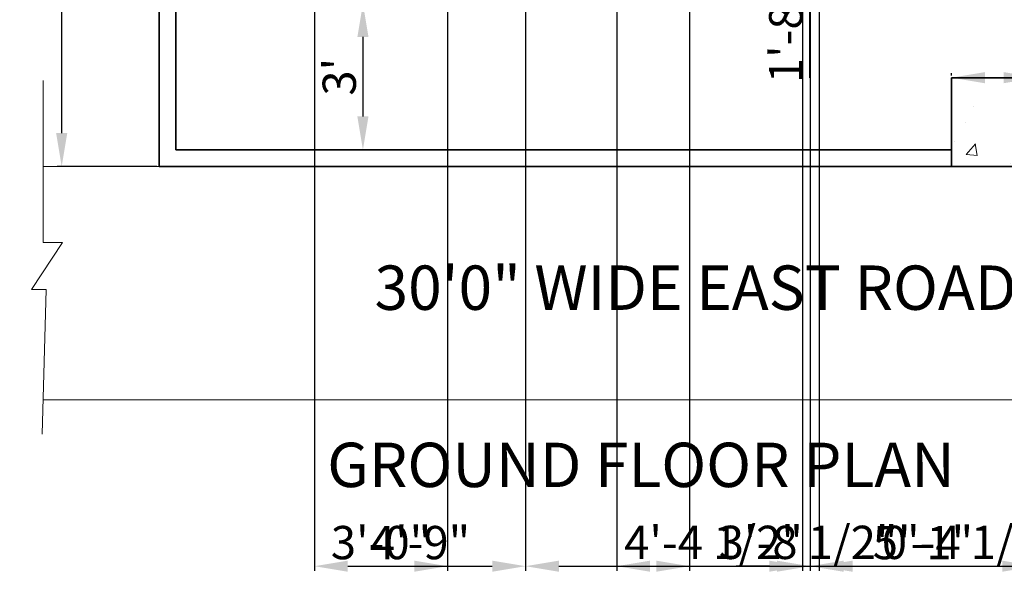
# Model space of a CAD drawing. Units: inches. Extents: x 53662 to 54269, y 37303 to 38048.
# Tile 1 of 6: x 53712 to 53979, y 37303 to 37459. Entities that reach past the tile are written whole.
import ezdxf

# ---------------------------------------------------------------- set-up
doc = ezdxf.new("R2010")
doc.units = ezdxf.units.IN
for name, color, linetype, lineweight in [('A-ANNO-DIMS', 2, 'Continuous', 18), ('A-ANNO-TEXT', 7, 'Continuous', 25), ('C-PROP', 7, 'Continuous', 35), ('C-ROAD', 8, 'Continuous', 18), ('C-SITE-PATT', 8, 'Continuous', 13)]:
    doc.layers.add(name, color=color, linetype=linetype, lineweight=lineweight)
doc.styles.get("Standard").update_dxf_attribs({"font": 'arial.ttf'})
doc.dimstyles.new('ISO-25', dxfattribs={"dimtxt": 9, "dimasz": 9, "dimexe": 1.25, "dimexo": 0.625, "dimtad": 1, "dimdec": 1, "dimrnd": 9, "dimlunit": 3, "dimtxsty": 'Standard', "dimcen": 2.5, "dimadec": 0, "dimazin": 0, "dimtfac": 1, "dimtdec": 1, "dimtmove": 0, "dimatfit": 3, "dimfxl": 1, "dimarcsym": 0})

# ---------------------------------------------------------------- blocks, each defined once
blk = doc.blocks.new('*D13')
at = {"layer": 'A-ANNO-DIMS', "color": 0, "lineweight": -2, "transparency": 16777216}
for p, q in [((53749.49, 37994.86), (53722.52, 37994.86)), ((53723.77, 37427.86), (53723.77, 37985.86)), ((53749.49, 37418.86), (53722.52, 37418.86))]:
    blk.add_line(p, q, dxfattribs=at)
at = {"layer": 'A-ANNO-DIMS', "color": 0, "transparency": 16777216}
for points in [[(53722.27, 37985.86), (53725.27, 37985.86), (53723.77, 37994.86)], [(53722.27, 37427.86), (53725.27, 37427.86), (53723.77, 37418.86)]]:
    blk.add_solid(points, dxfattribs=at)
at = {"layer": 'Defpoints', "color": 0, "transparency": 16777216}
for p in [(53723.77, 37994.86), (53750.11, 37994.86), (53750.11, 37418.86)]:
    blk.add_point(p, dxfattribs=at)
at = {"layer": 'A-ANNO-DIMS', "color": 0, "transparency": 16777216, "insert": (53718.55, 37706.86), "char_height": 9, "attachment_point": 5, "rotation": 90}
blk.add_mtext("48'", dxfattribs=at)
blk = doc.blocks.new('*D18')
at = {"layer": 'A-ANNO-DIMS', "color": 0, "lineweight": -2, "transparency": 16777216}
for p, q in [((53783.74, 37462.86), (53806.47, 37462.86)), ((53805.22, 37453.86), (53805.22, 37432.36)), ((53783.74, 37423.36), (53806.47, 37423.36))]:
    blk.add_line(p, q, dxfattribs=at)
at = {"layer": 'A-ANNO-DIMS', "color": 0, "transparency": 16777216}
for points in [[(53803.72, 37453.86), (53806.72, 37453.86), (53805.22, 37462.86)], [(53803.72, 37432.36), (53806.72, 37432.36), (53805.22, 37423.36)]]:
    blk.add_solid(points, dxfattribs=at)
at = {"layer": 'Defpoints', "color": 0, "transparency": 16777216}
for p in [(53783.11, 37462.86), (53783.11, 37423.36), (53805.22, 37423.36)]:
    blk.add_point(p, dxfattribs=at)
at = {"layer": 'A-ANNO-DIMS', "color": 0, "transparency": 16777216, "insert": (53799.99, 37443.11), "char_height": 9, "attachment_point": 5, "rotation": 90}
blk.add_mtext("3'", dxfattribs=at)
blk = doc.blocks.new('*D19')
at = {"layer": 'A-ANNO-DIMS', "color": 0, "lineweight": -2, "transparency": 16777216}
for p, q in [((53964.39, 37443.48), (53964.39, 37444.1)), ((53973.39, 37442.85), (53978.47, 37442.85)), ((53987.47, 37442.85), (54021.8, 37442.85)), ((53987.47, 37442.23), (53987.47, 37441.6))]:
    blk.add_line(p, q, dxfattribs=at)
at = {"layer": 'A-ANNO-DIMS', "color": 0, "transparency": 16777216}
for points in [[(53973.39, 37444.35), (53973.39, 37441.35), (53964.39, 37442.85)], [(53978.47, 37444.35), (53978.47, 37441.35), (53987.47, 37442.85)]]:
    blk.add_solid(points, dxfattribs=at)
at = {"layer": 'Defpoints', "color": 0, "transparency": 16777216}
for p in [(53964.39, 37442.85), (53987.47, 37442.85), (53987.47, 37442.85)]:
    blk.add_point(p, dxfattribs=at)
at = {"layer": 'A-ANNO-DIMS', "color": 0, "transparency": 16777216, "insert": (54009.13, 37448.08), "char_height": 9, "attachment_point": 5}
blk.add_mtext('2\'-3"', dxfattribs=at)
blk = doc.blocks.new('*D45')
at = {"layer": 'A-ANNO-DIMS', "color": 0, "lineweight": -2, "transparency": 16777216}
for p, q in [((53929.81, 37496.1), (53924.68, 37496.1)), ((53925.93, 37487.1), (53925.93, 37485.1)), ((53929.81, 37476.1), (53924.68, 37476.1)), ((53925.93, 37476.1), (53925.93, 37442.77))]:
    blk.add_line(p, q, dxfattribs=at)
at = {"layer": 'A-ANNO-DIMS', "color": 0, "transparency": 16777216}
for points in [[(53924.43, 37487.1), (53927.43, 37487.1), (53925.93, 37496.1)], [(53924.43, 37485.1), (53927.43, 37485.1), (53925.93, 37476.1)]]:
    blk.add_solid(points, dxfattribs=at)
at = {"layer": 'Defpoints', "color": 0, "transparency": 16777216}
for p in [(53930.43, 37496.1), (53925.93, 37476.1), (53930.43, 37476.1)]:
    blk.add_point(p, dxfattribs=at)
at = {"layer": 'A-ANNO-DIMS', "color": 0, "transparency": 16777216, "insert": (53920.71, 37454.94), "char_height": 9, "attachment_point": 5, "rotation": 90}
blk.add_mtext('1\'-8"', dxfattribs=at)
blk = doc.blocks.new('*D52')
at = {"layer": 'A-ANNO-DIMS', "color": 0, "lineweight": -2, "transparency": 16777216}
for p, q in [((53792.11, 37660.24), (53792.11, 37309.49)), ((53828.11, 37660.24), (53828.11, 37309.49)), ((53801.11, 37310.74), (53819.11, 37310.74))]:
    blk.add_line(p, q, dxfattribs=at)
at = {"layer": 'A-ANNO-DIMS', "color": 0, "transparency": 16777216}
for points in [[(53801.11, 37312.24), (53801.11, 37309.24), (53792.11, 37310.74)], [(53819.11, 37312.24), (53819.11, 37309.24), (53828.11, 37310.74)]]:
    blk.add_solid(points, dxfattribs=at)
at = {"layer": 'Defpoints', "color": 0, "transparency": 16777216}
for p in [(53792.11, 37660.86), (53828.11, 37660.86), (53828.11, 37310.74)]:
    blk.add_point(p, dxfattribs=at)
at = {"layer": 'A-ANNO-DIMS', "color": 0, "transparency": 16777216, "insert": (53810.11, 37315.96), "char_height": 9, "attachment_point": 5}
blk.add_mtext('3\'-0"', dxfattribs=at)
blk = doc.blocks.new('*D54')
at = {"layer": 'A-ANNO-DIMS', "color": 0, "lineweight": -2, "transparency": 16777216}
for p, q in [((53792.11, 37952.24), (53792.11, 37309.49)), ((53849.2, 37952.24), (53849.2, 37309.49)), ((53801.11, 37310.74), (53840.2, 37310.74))]:
    blk.add_line(p, q, dxfattribs=at)
at = {"layer": 'A-ANNO-DIMS', "color": 0, "transparency": 16777216}
for points in [[(53801.11, 37312.24), (53801.11, 37309.24), (53792.11, 37310.74)], [(53840.2, 37312.24), (53840.2, 37309.24), (53849.2, 37310.74)]]:
    blk.add_solid(points, dxfattribs=at)
at = {"layer": 'Defpoints', "color": 0, "transparency": 16777216}
for p in [(53792.11, 37952.86), (53849.2, 37952.86), (53849.2, 37310.74)]:
    blk.add_point(p, dxfattribs=at)
at = {"layer": 'A-ANNO-DIMS', "color": 0, "transparency": 16777216, "insert": (53820.66, 37315.96), "char_height": 9, "attachment_point": 5}
blk.add_mtext('4\'-9"', dxfattribs=at)
blk = doc.blocks.new('*D55')
at = {"layer": 'A-ANNO-DIMS', "color": 0, "lineweight": -2, "transparency": 16777216}
for p, q in [((53849.2, 37952.24), (53849.2, 37309.49)), ((53893.52, 37952.24), (53893.52, 37309.49)), ((53858.2, 37310.74), (53884.52, 37310.74)), ((53893.52, 37310.74), (53948.66, 37310.74))]:
    blk.add_line(p, q, dxfattribs=at)
at = {"layer": 'A-ANNO-DIMS', "color": 0, "transparency": 16777216}
for points in [[(53858.2, 37312.24), (53858.2, 37309.24), (53849.2, 37310.74)], [(53884.52, 37312.24), (53884.52, 37309.24), (53893.52, 37310.74)]]:
    blk.add_solid(points, dxfattribs=at)
at = {"layer": 'Defpoints', "color": 0, "transparency": 16777216}
for p in [(53849.2, 37952.86), (53893.52, 37952.86), (53893.52, 37310.74)]:
    blk.add_point(p, dxfattribs=at)
at = {"layer": 'A-ANNO-DIMS', "color": 0, "transparency": 16777216, "insert": (53925.59, 37316.02), "char_height": 9, "attachment_point": 5}
blk.add_mtext('3\'-8 1/2"', dxfattribs=at)
blk = doc.blocks.new('*D60')
at = {"layer": 'A-ANNO-DIMS', "color": 0, "lineweight": -2, "transparency": 16777216}
for p, q in [((53924.11, 37790.24), (53924.11, 37309.49)), ((53928.61, 37790.24), (53928.61, 37309.49)), ((53915.11, 37310.74), (53906.11, 37310.74)), ((53924.11, 37310.74), (53928.61, 37310.74)), ((53937.61, 37310.74), (53992.76, 37310.74))]:
    blk.add_line(p, q, dxfattribs=at)
at = {"layer": 'A-ANNO-DIMS', "color": 0, "transparency": 16777216}
for points in [[(53915.11, 37312.24), (53915.11, 37309.24), (53924.11, 37310.74)], [(53937.61, 37312.24), (53937.61, 37309.24), (53928.61, 37310.74)]]:
    blk.add_solid(points, dxfattribs=at)
at = {"layer": 'Defpoints', "color": 0, "transparency": 16777216}
for p in [(53924.11, 37790.86), (53928.61, 37790.86), (53928.61, 37310.74)]:
    blk.add_point(p, dxfattribs=at)
at = {"layer": 'A-ANNO-DIMS', "color": 0, "transparency": 16777216, "insert": (53969.69, 37316.02), "char_height": 9, "attachment_point": 5}
blk.add_mtext('0\'-4 1/2"', dxfattribs=at)
blk = doc.blocks.new('*D70')
at = {"layer": 'A-ANNO-DIMS', "color": 0, "lineweight": -2, "transparency": 16777216}
for p, q in [((53873.85, 37462.24), (53873.85, 37309.49)), ((53926.17, 37462.24), (53926.17, 37309.49)), ((53882.85, 37310.74), (53917.17, 37310.74))]:
    blk.add_line(p, q, dxfattribs=at)
at = {"layer": 'A-ANNO-DIMS', "color": 0, "transparency": 16777216}
for points in [[(53882.85, 37312.24), (53882.85, 37309.24), (53873.85, 37310.74)], [(53917.17, 37312.24), (53917.17, 37309.24), (53926.17, 37310.74)]]:
    blk.add_solid(points, dxfattribs=at)
at = {"layer": 'Defpoints', "color": 0, "transparency": 16777216}
for p in [(53873.85, 37462.86), (53926.17, 37462.86), (53926.17, 37310.74)]:
    blk.add_point(p, dxfattribs=at)
at = {"layer": 'A-ANNO-DIMS', "color": 0, "transparency": 16777216, "insert": (53900.01, 37316.02), "char_height": 9, "attachment_point": 5}
blk.add_mtext('4\'-4 1/2"', dxfattribs=at)
blk = doc.blocks.new('*D71')
at = {"layer": 'A-ANNO-DIMS', "color": 0, "lineweight": -2, "transparency": 16777216}
for p, q in [((53926.17, 37462.24), (53926.17, 37309.49)), ((53987.11, 37462.24), (53987.11, 37309.49)), ((53935.17, 37310.74), (53978.11, 37310.74))]:
    blk.add_line(p, q, dxfattribs=at)
at = {"layer": 'A-ANNO-DIMS', "color": 0, "transparency": 16777216}
for points in [[(53935.17, 37312.24), (53935.17, 37309.24), (53926.17, 37310.74)], [(53978.11, 37312.24), (53978.11, 37309.24), (53987.11, 37310.74)]]:
    blk.add_solid(points, dxfattribs=at)
at = {"layer": 'Defpoints', "color": 0, "transparency": 16777216}
for p in [(53926.17, 37462.86), (53987.11, 37462.86), (53987.11, 37310.74)]:
    blk.add_point(p, dxfattribs=at)
at = {"layer": 'A-ANNO-DIMS', "color": 0, "transparency": 16777216, "insert": (53956.64, 37315.96), "char_height": 9, "attachment_point": 5}
blk.add_mtext('5\'-1"', dxfattribs=at)

msp = doc.modelspace()

# ---------------------------------------------------------------- hatches: boundary and pattern name
at = {"layer": 'C-SITE-PATT'}
h = msp.add_hatch(dxfattribs=at)
h.set_pattern_fill('AR-CONC', color=256, scale=0.2)
h.paths.add_polyline_path([(54182.11, 37442.85), (54163.41, 37442.85), (54163.41, 37418.86), (54182.11, 37418.86)])
h.paths.add_polyline_path([(53987.47, 37442.85), (53964.39, 37442.85), (53964.39, 37418.86), (53987.47, 37418.86)])

# ---------------------------------------------------------------- linework, layer by layer
at = {"layer": 'C-PROP'}
for p, q in [((53750.11, 37418.86), (53750.11, 37615.86)), ((53754.61, 37423.36), (53754.61, 37615.86)), ((53987.47, 37442.85), (53964.39, 37442.85)), ((53964.39, 37442.85), (53964.39, 37418.86)), ((53754.61, 37423.36), (53964.39, 37423.36)), ((53750.11, 37418.86), (54182.11, 37418.86))]:
    msp.add_line(p, q, dxfattribs=at)
at = {"layer": 'C-ROAD'}
for p, q in [((53718.77, 37442.1), (53718.77, 37398.28)), ((53750.11, 37418.86), (53718.77, 37418.86)), ((53723.96, 37398.28), (53715.6, 37385.54)), ((53718.77, 37398.28), (53723.96, 37398.28)), ((53715.6, 37385.54), (53719.53, 37385.55)), ((53719.53, 37385.55), (53718.49, 37346.47)), ((53718.77, 37355.76), (54220.88, 37355.76))]:
    msp.add_line(p, q, dxfattribs=at)

# ---------------------------------------------------------------- texts
at = {"layer": 'A-ANNO-TEXT', "char_height": 12, "attachment_point": 1}
for s, width, insert in [('30\'0" WIDE EAST ROAD', 314.7476, (53808.35, 37392.06)), ('GROUND FLOOR PLAN', 335.4467, (53795.57, 37344.14))]:
    msp.add_mtext_dynamic_manual_height_columns(s, width=width, gutter_width=12.5, heights=[0], dxfattribs=dict(at, insert=insert))

# ---------------------------------------------------------------- dimensions: what is measured, and where the dimension line sits
at = {"layer": 'A-ANNO-DIMS'}
for base, p1, p2, angle, override, picture, middle in [((53723.77, 37994.86), (53750.11, 37418.86), (53750.11, 37994.86), 90, {"dimclrd": 0, "dimclre": 0, "dimclrt": 0}, '*D13', (53718.55, 37706.86)), ((53925.93, 37476.1), (53930.43, 37496.1), (53930.43, 37476.1), 270, {"dimdec": 1, "dimlfac": 1, "dimrnd": 0, "dimzin": 1, "dimdsep": 46, "dimlunit": 4, "dimfrac": 2}, '*D45', (53920.71, 37454.94))]:
    dim = msp.add_linear_dim(base=base, p1=p1, p2=p2, angle=angle, dimstyle='ISO-25', override=override, dxfattribs=at)
    dim.commit()
    dim.dimension.update_dxf_attribs({"geometry": picture, "text_midpoint": middle})
for base, p1, p2, override, picture, middle in [((53849.2, 37310.74), (53792.11, 37952.86), (53849.2, 37952.86), {"dimdec": 1, "dimlfac": 1, "dimrnd": 0, "dimzin": 1, "dimdsep": 46, "dimlunit": 4, "dimfrac": 2}, '*D54', (53820.66, 37315.96)), ((53893.52, 37310.74), (53849.2, 37952.86), (53893.52, 37952.86), {"dimdec": 1, "dimlfac": 1, "dimrnd": 0, "dimzin": 1, "dimdsep": 46, "dimlunit": 4, "dimfrac": 2}, '*D55', (53925.59, 37316.02)), ((53928.61, 37310.74), (53924.11, 37790.86), (53928.61, 37790.86), {"dimdec": 1, "dimlfac": 1, "dimrnd": 0, "dimzin": 1, "dimdsep": 46, "dimlunit": 4, "dimfrac": 2}, '*D60', (53969.69, 37316.02)), ((53828.11, 37310.74), (53792.11, 37660.86), (53828.11, 37660.86), {"dimdec": 1, "dimlfac": 1, "dimrnd": 0, "dimzin": 1, "dimdsep": 46, "dimlunit": 4, "dimfrac": 2}, '*D52', (53810.11, 37315.96)), ((53926.17, 37310.74), (53873.85, 37462.86), (53926.17, 37462.86), {"dimdec": 1, "dimlfac": 1, "dimrnd": 0, "dimzin": 1, "dimdsep": 46, "dimlunit": 4, "dimfrac": 2}, '*D70', (53900.01, 37316.02)), ((53987.11, 37310.74), (53926.17, 37462.86), (53987.11, 37462.86), {"dimdec": 1, "dimlfac": 1, "dimrnd": 0, "dimzin": 1, "dimdsep": 46, "dimlunit": 4, "dimfrac": 2}, '*D71', (53956.64, 37315.96)), ((53987.47, 37442.85), (53964.39, 37442.85), (53987.47, 37442.85), {"dimclrd": 0, "dimclre": 0, "dimclrt": 0}, '*D19', (54009.13, 37448.08))]:
    dim = msp.add_linear_dim(base=base, p1=p1, p2=p2, dimstyle='ISO-25', override=override, dxfattribs=at)
    dim.commit()
    dim.dimension.update_dxf_attribs({"geometry": picture, "text_midpoint": middle})
dim = msp.add_aligned_dim(p1=(53783.11, 37462.86), p2=(53783.11, 37423.36), distance=22.1, dimstyle='ISO-25', override={"dimclrd": 0, "dimclre": 0, "dimclrt": 0}, dxfattribs=at)
dim.commit()
dim.dimension.update_dxf_attribs({"geometry": '*D18', "text_midpoint": (53799.99, 37443.11)})

doc.saveas('drawing.dxf')
